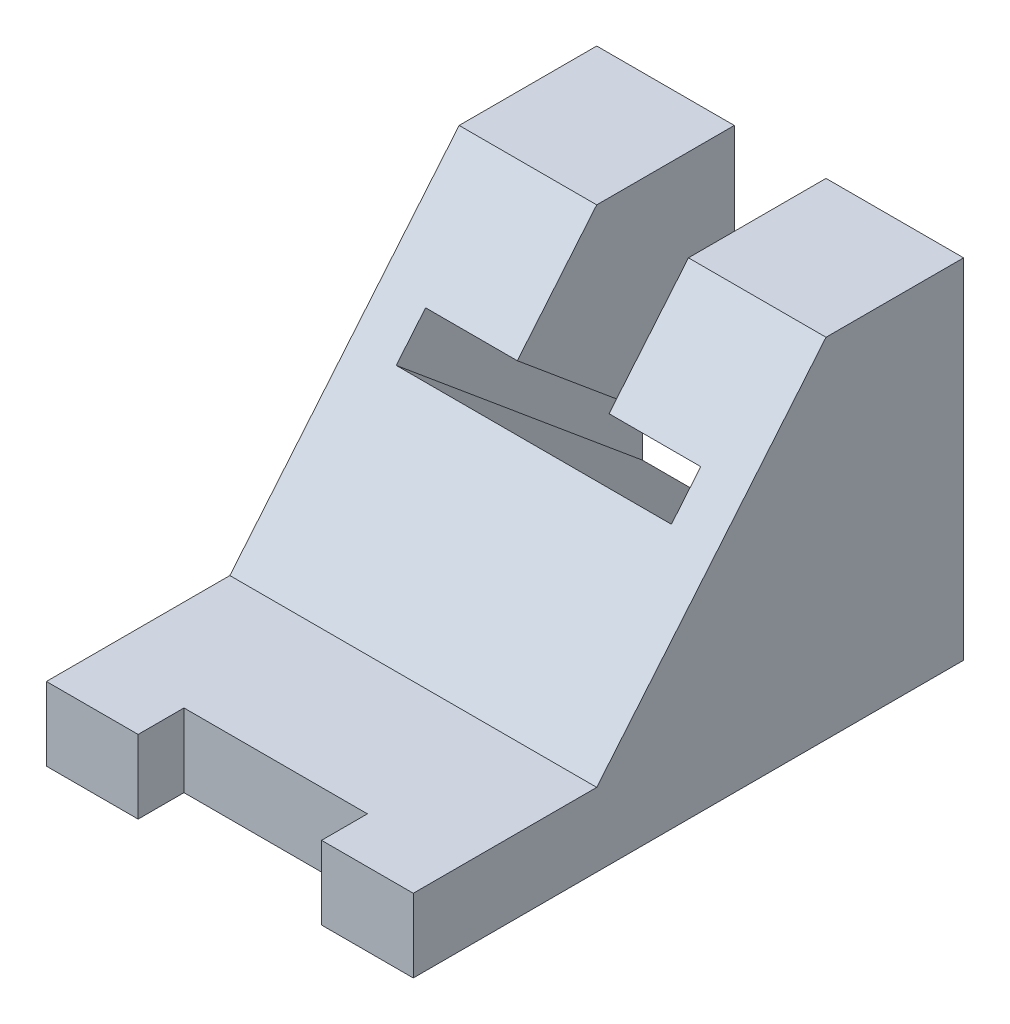
ISO-10303-21;
HEADER;
FILE_DESCRIPTION(('STEP AP214'),'2;1');
FILE_NAME('part.step','',(''),(''),'','','');
FILE_SCHEMA(('AUTOMOTIVE_DESIGN { 1 0 10303 214 1 1 1 1 }'));
ENDSEC;
DATA;
#1=APPLICATION_CONTEXT('core data for automotive mechanical design processes');
#2=APPLICATION_PROTOCOL_DEFINITION('international standard','automotive_design',2000,#1);
#3=PRODUCT_CONTEXT('',#1,'mechanical');
#4=PRODUCT('Part','Part','',(#3));
#5=PRODUCT_RELATED_PRODUCT_CATEGORY('part','',(#4));
#6=PRODUCT_DEFINITION_FORMATION('','',#4);
#7=PRODUCT_DEFINITION_CONTEXT('part definition',#1,'design');
#8=PRODUCT_DEFINITION('design','',#6,#7);
#9=PRODUCT_DEFINITION_SHAPE('','',#8);
#10=(LENGTH_UNIT() NAMED_UNIT(*) SI_UNIT(.MILLI.,.METRE.));
#11=(NAMED_UNIT(*) PLANE_ANGLE_UNIT() SI_UNIT($,.RADIAN.));
#12=(NAMED_UNIT(*) SI_UNIT($,.STERADIAN.) SOLID_ANGLE_UNIT());
#13=UNCERTAINTY_MEASURE_WITH_UNIT(LENGTH_MEASURE(1.E-05),#10,'distance_accuracy_value','');
#14=(GEOMETRIC_REPRESENTATION_CONTEXT(3) GLOBAL_UNCERTAINTY_ASSIGNED_CONTEXT((#13)) GLOBAL_UNIT_ASSIGNED_CONTEXT((#10,
#11,#12)) REPRESENTATION_CONTEXT('',''));
#15=CARTESIAN_POINT('',(0.,0.,0.));
#16=DIRECTION('',(0.,0.,1.));
#17=DIRECTION('',(1.,0.,0.));
#18=AXIS2_PLACEMENT_3D('',#15,#16,#17);
#19=CARTESIAN_POINT('',(-20.,38.,-30.));
#20=DIRECTION('',(0.,1.,0.));
#21=DIRECTION('',(0.,0.,1.));
#22=AXIS2_PLACEMENT_3D('',#19,#20,#21);
#23=PLANE('',#22);
#24=DIRECTION('',(0.,0.,-1.));
#25=VECTOR('',#24,1.);
#26=CARTESIAN_POINT('',(5.,38.,-15.));
#27=LINE('',#26,#25);
#28=CARTESIAN_POINT('',(5.,38.,-15.));
#29=VERTEX_POINT('',#28);
#30=CARTESIAN_POINT('',(5.,38.,-30.));
#31=VERTEX_POINT('',#30);
#32=EDGE_CURVE('E187',#29,#31,#27,.T.);
#33=ORIENTED_EDGE('',*,*,#32,.F.);
#34=DIRECTION('',(1.,0.,0.));
#35=VECTOR('',#34,1.);
#36=CARTESIAN_POINT('',(-20.,38.,-15.));
#37=LINE('',#36,#35);
#38=CARTESIAN_POINT('',(20.,38.,-15.));
#39=VERTEX_POINT('',#38);
#40=EDGE_CURVE('E275',#29,#39,#37,.T.);
#41=ORIENTED_EDGE('',*,*,#40,.T.);
#42=DIRECTION('',(0.,0.,1.));
#43=VECTOR('',#42,1.);
#44=CARTESIAN_POINT('',(20.,38.,-30.));
#45=LINE('',#44,#43);
#46=CARTESIAN_POINT('',(20.,38.,-30.));
#47=VERTEX_POINT('',#46);
#48=EDGE_CURVE('E269',#47,#39,#45,.T.);
#49=ORIENTED_EDGE('',*,*,#48,.F.);
#50=DIRECTION('',(1.,0.,0.));
#51=VECTOR('',#50,1.);
#52=CARTESIAN_POINT('',(-20.,38.,-30.));
#53=LINE('',#52,#51);
#54=EDGE_CURVE('E195',#31,#47,#53,.T.);
#55=ORIENTED_EDGE('',*,*,#54,.F.);
#56=EDGE_LOOP('',(#33,#41,#49,#55));
#57=FACE_BOUND('',#56,.T.);
#58=ADVANCED_FACE('F39',(#57),#23,.T.);
#59=CARTESIAN_POINT('',(20.,8.,30.));
#60=DIRECTION('',(0.,0.,-1.));
#61=DIRECTION('',(-1.,0.,0.));
#62=AXIS2_PLACEMENT_3D('',#59,#60,#61);
#63=PLANE('',#62);
#64=DIRECTION('',(1.,0.,0.));
#65=VECTOR('',#64,1.);
#66=CARTESIAN_POINT('',(20.,8.,30.));
#67=LINE('',#66,#65);
#68=CARTESIAN_POINT('',(10.,8.,30.));
#69=VERTEX_POINT('',#68);
#70=CARTESIAN_POINT('',(20.,8.,30.));
#71=VERTEX_POINT('',#70);
#72=EDGE_CURVE('E217',#69,#71,#67,.T.);
#73=ORIENTED_EDGE('',*,*,#72,.F.);
#74=DIRECTION('',(0.,1.,0.));
#75=VECTOR('',#74,1.);
#76=CARTESIAN_POINT('',(10.,-12.,30.));
#77=LINE('',#76,#75);
#78=CARTESIAN_POINT('',(10.,0.,30.));
#79=VERTEX_POINT('',#78);
#80=EDGE_CURVE('E210',#79,#69,#77,.T.);
#81=ORIENTED_EDGE('',*,*,#80,.F.);
#82=DIRECTION('',(1.,0.,0.));
#83=VECTOR('',#82,1.);
#84=CARTESIAN_POINT('',(20.,0.,30.));
#85=LINE('',#84,#83);
#86=CARTESIAN_POINT('',(20.,0.,30.));
#87=VERTEX_POINT('',#86);
#88=EDGE_CURVE('E226',#79,#87,#85,.T.);
#89=ORIENTED_EDGE('',*,*,#88,.T.);
#90=DIRECTION('',(0.,-1.,0.));
#91=VECTOR('',#90,1.);
#92=CARTESIAN_POINT('',(20.,8.,30.));
#93=LINE('',#92,#91);
#94=EDGE_CURVE('E237',#71,#87,#93,.T.);
#95=ORIENTED_EDGE('',*,*,#94,.F.);
#96=EDGE_LOOP('',(#73,#81,#89,#95));
#97=FACE_BOUND('',#96,.T.);
#98=ADVANCED_FACE('F342',(#97),#63,.F.);
#99=CARTESIAN_POINT('',(-20.,8.,30.));
#100=DIRECTION('',(1.,0.,0.));
#101=DIRECTION('',(0.,0.,-1.));
#102=AXIS2_PLACEMENT_3D('',#99,#100,#101);
#103=PLANE('',#102);
#104=DIRECTION('',(0.,0.,1.));
#105=VECTOR('',#104,1.);
#106=CARTESIAN_POINT('',(-20.,8.,30.));
#107=LINE('',#106,#105);
#108=CARTESIAN_POINT('',(-20.,8.,9.99999999999999));
#109=VERTEX_POINT('',#108);
#110=CARTESIAN_POINT('',(-20.,8.,30.));
#111=VERTEX_POINT('',#110);
#112=EDGE_CURVE('E216',#109,#111,#107,.T.);
#113=ORIENTED_EDGE('',*,*,#112,.F.);
#114=DIRECTION('',(0.,0.768221279597376,-0.64018439966448));
#115=VECTOR('',#114,1.);
#116=CARTESIAN_POINT('',(-20.,38.,-15.));
#117=LINE('',#116,#115);
#118=CARTESIAN_POINT('',(-20.,38.,-15.));
#119=VERTEX_POINT('',#118);
#120=EDGE_CURVE('E276',#109,#119,#117,.T.);
#121=ORIENTED_EDGE('',*,*,#120,.T.);
#122=DIRECTION('',(0.,0.,1.));
#123=VECTOR('',#122,1.);
#124=CARTESIAN_POINT('',(-20.,38.,-30.));
#125=LINE('',#124,#123);
#126=CARTESIAN_POINT('',(-20.,38.,-30.));
#127=VERTEX_POINT('',#126);
#128=EDGE_CURVE('E196',#127,#119,#125,.T.);
#129=ORIENTED_EDGE('',*,*,#128,.F.);
#130=DIRECTION('',(0.,-1.,0.));
#131=VECTOR('',#130,1.);
#132=CARTESIAN_POINT('',(-20.,8.,-30.));
#133=LINE('',#132,#131);
#134=CARTESIAN_POINT('',(-20.,0.,-30.));
#135=VERTEX_POINT('',#134);
#136=EDGE_CURVE('E188',#127,#135,#133,.T.);
#137=ORIENTED_EDGE('',*,*,#136,.T.);
#138=DIRECTION('',(0.,0.,1.));
#139=VECTOR('',#138,1.);
#140=CARTESIAN_POINT('',(-20.,0.,30.));
#141=LINE('',#140,#139);
#142=CARTESIAN_POINT('',(-20.,0.,30.));
#143=VERTEX_POINT('',#142);
#144=EDGE_CURVE('E209',#135,#143,#141,.T.);
#145=ORIENTED_EDGE('',*,*,#144,.T.);
#146=DIRECTION('',(0.,-1.,0.));
#147=VECTOR('',#146,1.);
#148=CARTESIAN_POINT('',(-20.,8.,30.));
#149=LINE('',#148,#147);
#150=EDGE_CURVE('E245',#111,#143,#149,.T.);
#151=ORIENTED_EDGE('',*,*,#150,.F.);
#152=EDGE_LOOP('',(#113,#121,#129,#137,#145,#151));
#153=FACE_BOUND('',#152,.T.);
#154=ADVANCED_FACE('F41',(#153),#103,.F.);
#155=CARTESIAN_POINT('',(-10.,0.,30.));
#156=VERTEX_POINT('',#155);
#157=EDGE_CURVE('E230',#143,#156,#85,.T.);
#158=ORIENTED_EDGE('',*,*,#157,.T.);
#159=DIRECTION('',(0.,1.,0.));
#160=VECTOR('',#159,1.);
#161=CARTESIAN_POINT('',(-10.,-12.,30.));
#162=LINE('',#161,#160);
#163=CARTESIAN_POINT('',(-10.,8.,30.));
#164=VERTEX_POINT('',#163);
#165=EDGE_CURVE('E208',#156,#164,#162,.T.);
#166=ORIENTED_EDGE('',*,*,#165,.T.);
#167=EDGE_CURVE('E219',#111,#164,#67,.T.);
#168=ORIENTED_EDGE('',*,*,#167,.F.);
#169=ORIENTED_EDGE('',*,*,#150,.T.);
#170=EDGE_LOOP('',(#158,#166,#168,#169));
#171=FACE_BOUND('',#170,.T.);
#172=ADVANCED_FACE('F253',(#171),#63,.F.);
#173=CARTESIAN_POINT('',(20.,8.,30.));
#174=DIRECTION('',(-1.,0.,0.));
#175=DIRECTION('',(0.,0.,1.));
#176=AXIS2_PLACEMENT_3D('',#173,#174,#175);
#177=PLANE('',#176);
#178=ORIENTED_EDGE('',*,*,#48,.T.);
#179=DIRECTION('',(0.,0.768221279597376,-0.64018439966448));
#180=VECTOR('',#179,1.);
#181=CARTESIAN_POINT('',(20.,38.,-15.));
#182=LINE('',#181,#180);
#183=CARTESIAN_POINT('',(20.,8.,9.99999999999999));
#184=VERTEX_POINT('',#183);
#185=EDGE_CURVE('E280',#184,#39,#182,.T.);
#186=ORIENTED_EDGE('',*,*,#185,.F.);
#187=DIRECTION('',(0.,0.,-1.));
#188=VECTOR('',#187,1.);
#189=CARTESIAN_POINT('',(20.,8.,30.));
#190=LINE('',#189,#188);
#191=EDGE_CURVE('E221',#71,#184,#190,.T.);
#192=ORIENTED_EDGE('',*,*,#191,.F.);
#193=ORIENTED_EDGE('',*,*,#94,.T.);
#194=DIRECTION('',(0.,0.,-1.));
#195=VECTOR('',#194,1.);
#196=CARTESIAN_POINT('',(20.,0.,30.));
#197=LINE('',#196,#195);
#198=CARTESIAN_POINT('',(20.,0.,-30.));
#199=VERTEX_POINT('',#198);
#200=EDGE_CURVE('E235',#87,#199,#197,.T.);
#201=ORIENTED_EDGE('',*,*,#200,.T.);
#202=DIRECTION('',(0.,-1.,0.));
#203=VECTOR('',#202,1.);
#204=CARTESIAN_POINT('',(20.,8.,-30.));
#205=LINE('',#204,#203);
#206=EDGE_CURVE('E236',#47,#199,#205,.T.);
#207=ORIENTED_EDGE('',*,*,#206,.F.);
#208=EDGE_LOOP('',(#178,#186,#192,#193,#201,#207));
#209=FACE_BOUND('',#208,.T.);
#210=ADVANCED_FACE('F270',(#209),#177,.F.);
#211=CARTESIAN_POINT('',(20.,8.,-30.));
#212=DIRECTION('',(0.,0.,1.));
#213=DIRECTION('',(1.,0.,0.));
#214=AXIS2_PLACEMENT_3D('',#211,#212,#213);
#215=PLANE('',#214);
#216=DIRECTION('',(0.,1.,0.));
#217=VECTOR('',#216,1.);
#218=CARTESIAN_POINT('',(5.,8.,-30.));
#219=LINE('',#218,#217);
#220=CARTESIAN_POINT('',(5.,7.8976526277451,-30.));
#221=VERTEX_POINT('',#220);
#222=EDGE_CURVE('E176',#221,#31,#219,.T.);
#223=ORIENTED_EDGE('',*,*,#222,.T.);
#224=ORIENTED_EDGE('',*,*,#54,.T.);
#225=ORIENTED_EDGE('',*,*,#206,.T.);
#226=DIRECTION('',(-1.,0.,0.));
#227=VECTOR('',#226,1.);
#228=CARTESIAN_POINT('',(20.,0.,-30.));
#229=LINE('',#228,#227);
#230=EDGE_CURVE('E218',#199,#135,#229,.T.);
#231=ORIENTED_EDGE('',*,*,#230,.T.);
#232=ORIENTED_EDGE('',*,*,#136,.F.);
#233=CARTESIAN_POINT('',(-5.,38.,-30.));
#234=VERTEX_POINT('',#233);
#235=EDGE_CURVE('E182',#127,#234,#53,.T.);
#236=ORIENTED_EDGE('',*,*,#235,.T.);
#237=DIRECTION('',(0.,-1.,0.));
#238=VECTOR('',#237,1.);
#239=CARTESIAN_POINT('',(-5.,8.,-30.));
#240=LINE('',#239,#238);
#241=CARTESIAN_POINT('',(-5.,7.8976526277451,-30.));
#242=VERTEX_POINT('',#241);
#243=EDGE_CURVE('E164',#234,#242,#240,.T.);
#244=ORIENTED_EDGE('',*,*,#243,.T.);
#245=DIRECTION('',(-1.,0.,0.));
#246=VECTOR('',#245,1.);
#247=CARTESIAN_POINT('',(20.,7.89765262774512,-30.));
#248=LINE('',#247,#246);
#249=CARTESIAN_POINT('',(-15.,7.89765262774509,-30.));
#250=VERTEX_POINT('',#249);
#251=EDGE_CURVE('E174',#242,#250,#248,.T.);
#252=ORIENTED_EDGE('',*,*,#251,.T.);
#253=DIRECTION('',(0.,-1.,0.));
#254=VECTOR('',#253,1.);
#255=CARTESIAN_POINT('',(-15.,7.99999999999999,-30.));
#256=LINE('',#255,#254);
#257=CARTESIAN_POINT('',(-15.,1.38911123115622,-30.));
#258=VERTEX_POINT('',#257);
#259=EDGE_CURVE('E286',#250,#258,#256,.T.);
#260=ORIENTED_EDGE('',*,*,#259,.T.);
#261=DIRECTION('',(1.,0.,0.));
#262=VECTOR('',#261,1.);
#263=CARTESIAN_POINT('',(20.,1.38911123115622,-30.));
#264=LINE('',#263,#262);
#265=CARTESIAN_POINT('',(15.,1.38911123115622,-30.));
#266=VERTEX_POINT('',#265);
#267=EDGE_CURVE('E284',#258,#266,#264,.T.);
#268=ORIENTED_EDGE('',*,*,#267,.T.);
#269=DIRECTION('',(0.,1.,0.));
#270=VECTOR('',#269,1.);
#271=CARTESIAN_POINT('',(15.,8.,-30.));
#272=LINE('',#271,#270);
#273=CARTESIAN_POINT('',(15.,7.8976526277451,-30.));
#274=VERTEX_POINT('',#273);
#275=EDGE_CURVE('E278',#266,#274,#272,.T.);
#276=ORIENTED_EDGE('',*,*,#275,.T.);
#277=DIRECTION('',(-1.,0.,0.));
#278=VECTOR('',#277,1.);
#279=CARTESIAN_POINT('',(20.,7.8976526277451,-30.));
#280=LINE('',#279,#278);
#281=EDGE_CURVE('E291',#274,#221,#280,.T.);
#282=ORIENTED_EDGE('',*,*,#281,.T.);
#283=EDGE_LOOP('',(#223,#224,#225,#231,#232,#236,#244,#252,#260,#268,#276,#282));
#284=FACE_BOUND('',#283,.T.);
#285=ADVANCED_FACE('F189',(#284),#215,.F.);
#286=CARTESIAN_POINT('',(0.,8.,0.));
#287=DIRECTION('',(0.,1.,0.));
#288=DIRECTION('',(0.,0.,1.));
#289=AXIS2_PLACEMENT_3D('',#286,#287,#288);
#290=PLANE('',#289);
#291=DIRECTION('',(1.,0.,0.));
#292=VECTOR('',#291,1.);
#293=CARTESIAN_POINT('',(-20.,8.,9.99999999999999));
#294=LINE('',#293,#292);
#295=EDGE_CURVE('E192',#109,#184,#294,.T.);
#296=ORIENTED_EDGE('',*,*,#295,.F.);
#297=ORIENTED_EDGE('',*,*,#112,.T.);
#298=ORIENTED_EDGE('',*,*,#167,.T.);
#299=DIRECTION('',(0.,0.,1.));
#300=VECTOR('',#299,1.);
#301=CARTESIAN_POINT('',(-10.,8.,30.));
#302=LINE('',#301,#300);
#303=CARTESIAN_POINT('',(-10.,8.,25.));
#304=VERTEX_POINT('',#303);
#305=EDGE_CURVE('E204',#304,#164,#302,.T.);
#306=ORIENTED_EDGE('',*,*,#305,.F.);
#307=DIRECTION('',(-1.,0.,0.));
#308=VECTOR('',#307,1.);
#309=CARTESIAN_POINT('',(-10.,8.,25.));
#310=LINE('',#309,#308);
#311=CARTESIAN_POINT('',(10.,8.,25.));
#312=VERTEX_POINT('',#311);
#313=EDGE_CURVE('E203',#312,#304,#310,.T.);
#314=ORIENTED_EDGE('',*,*,#313,.F.);
#315=DIRECTION('',(0.,0.,-1.));
#316=VECTOR('',#315,1.);
#317=CARTESIAN_POINT('',(10.,8.,30.));
#318=LINE('',#317,#316);
#319=EDGE_CURVE('E191',#69,#312,#318,.T.);
#320=ORIENTED_EDGE('',*,*,#319,.F.);
#321=ORIENTED_EDGE('',*,*,#72,.T.);
#322=ORIENTED_EDGE('',*,*,#191,.T.);
#323=EDGE_LOOP('',(#296,#297,#298,#306,#314,#320,#321,#322));
#324=FACE_BOUND('',#323,.T.);
#325=ADVANCED_FACE('F334',(#324),#290,.T.);
#326=CARTESIAN_POINT('',(0.,0.,0.));
#327=DIRECTION('',(0.,1.,0.));
#328=DIRECTION('',(0.,0.,1.));
#329=AXIS2_PLACEMENT_3D('',#326,#327,#328);
#330=PLANE('',#329);
#331=ORIENTED_EDGE('',*,*,#88,.F.);
#332=DIRECTION('',(0.,0.,-1.));
#333=VECTOR('',#332,1.);
#334=CARTESIAN_POINT('',(10.,0.,0.));
#335=LINE('',#334,#333);
#336=CARTESIAN_POINT('',(10.,0.,25.));
#337=VERTEX_POINT('',#336);
#338=EDGE_CURVE('E11',#79,#337,#335,.T.);
#339=ORIENTED_EDGE('',*,*,#338,.T.);
#340=DIRECTION('',(-1.,0.,0.));
#341=VECTOR('',#340,1.);
#342=CARTESIAN_POINT('',(0.,0.,25.));
#343=LINE('',#342,#341);
#344=CARTESIAN_POINT('',(-10.,0.,25.));
#345=VERTEX_POINT('',#344);
#346=EDGE_CURVE('E244',#337,#345,#343,.T.);
#347=ORIENTED_EDGE('',*,*,#346,.T.);
#348=DIRECTION('',(0.,0.,1.));
#349=VECTOR('',#348,1.);
#350=CARTESIAN_POINT('',(-10.,0.,0.));
#351=LINE('',#350,#349);
#352=EDGE_CURVE('E50',#345,#156,#351,.T.);
#353=ORIENTED_EDGE('',*,*,#352,.T.);
#354=ORIENTED_EDGE('',*,*,#157,.F.);
#355=ORIENTED_EDGE('',*,*,#144,.F.);
#356=ORIENTED_EDGE('',*,*,#230,.F.);
#357=ORIENTED_EDGE('',*,*,#200,.F.);
#358=EDGE_LOOP('',(#331,#339,#347,#353,#354,#355,#356,#357));
#359=FACE_BOUND('',#358,.T.);
#360=ADVANCED_FACE('F252',(#359),#330,.F.);
#361=CARTESIAN_POINT('',(10.,-12.,30.));
#362=DIRECTION('',(1.,0.,0.));
#363=DIRECTION('',(0.,0.,-1.));
#364=AXIS2_PLACEMENT_3D('',#361,#362,#363);
#365=PLANE('',#364);
#366=ORIENTED_EDGE('',*,*,#80,.T.);
#367=ORIENTED_EDGE('',*,*,#319,.T.);
#368=DIRECTION('',(0.,1.,0.));
#369=VECTOR('',#368,1.);
#370=CARTESIAN_POINT('',(10.,-12.,25.));
#371=LINE('',#370,#369);
#372=EDGE_CURVE('E207',#337,#312,#371,.T.);
#373=ORIENTED_EDGE('',*,*,#372,.F.);
#374=ORIENTED_EDGE('',*,*,#338,.F.);
#375=EDGE_LOOP('',(#366,#367,#373,#374));
#376=FACE_BOUND('',#375,.T.);
#377=ADVANCED_FACE('F341',(#376),#365,.F.);
#378=CARTESIAN_POINT('',(-10.,-12.,30.));
#379=DIRECTION('',(-1.,0.,0.));
#380=DIRECTION('',(0.,0.,1.));
#381=AXIS2_PLACEMENT_3D('',#378,#379,#380);
#382=PLANE('',#381);
#383=DIRECTION('',(0.,1.,0.));
#384=VECTOR('',#383,1.);
#385=CARTESIAN_POINT('',(-10.,-12.,25.));
#386=LINE('',#385,#384);
#387=EDGE_CURVE('E214',#345,#304,#386,.T.);
#388=ORIENTED_EDGE('',*,*,#387,.T.);
#389=ORIENTED_EDGE('',*,*,#305,.T.);
#390=ORIENTED_EDGE('',*,*,#165,.F.);
#391=ORIENTED_EDGE('',*,*,#352,.F.);
#392=EDGE_LOOP('',(#388,#389,#390,#391));
#393=FACE_BOUND('',#392,.T.);
#394=ADVANCED_FACE('F347',(#393),#382,.F.);
#395=CARTESIAN_POINT('',(-10.,-12.,25.));
#396=DIRECTION('',(0.,0.,-1.));
#397=DIRECTION('',(-1.,0.,0.));
#398=AXIS2_PLACEMENT_3D('',#395,#396,#397);
#399=PLANE('',#398);
#400=ORIENTED_EDGE('',*,*,#372,.T.);
#401=ORIENTED_EDGE('',*,*,#313,.T.);
#402=ORIENTED_EDGE('',*,*,#387,.F.);
#403=ORIENTED_EDGE('',*,*,#346,.F.);
#404=EDGE_LOOP('',(#400,#401,#402,#403));
#405=FACE_BOUND('',#404,.T.);
#406=ADVANCED_FACE('F346',(#405),#399,.F.);
#407=DIRECTION('',(0.,0.,1.));
#408=VECTOR('',#407,1.);
#409=CARTESIAN_POINT('',(-5.,38.,-15.));
#410=LINE('',#409,#408);
#411=CARTESIAN_POINT('',(-5.,38.,-15.));
#412=VERTEX_POINT('',#411);
#413=EDGE_CURVE('E169',#234,#412,#410,.T.);
#414=ORIENTED_EDGE('',*,*,#413,.F.);
#415=ORIENTED_EDGE('',*,*,#235,.F.);
#416=ORIENTED_EDGE('',*,*,#128,.T.);
#417=EDGE_CURVE('E184',#119,#412,#37,.T.);
#418=ORIENTED_EDGE('',*,*,#417,.T.);
#419=EDGE_LOOP('',(#414,#415,#416,#418));
#420=FACE_BOUND('',#419,.T.);
#421=ADVANCED_FACE('F181',(#420),#23,.T.);
#422=CARTESIAN_POINT('',(-20.,38.,-15.));
#423=DIRECTION('',(0.,-0.64018439966448,-0.768221279597376));
#424=DIRECTION('',(0.,0.768221279597376,-0.64018439966448));
#425=AXIS2_PLACEMENT_3D('',#422,#423,#424);
#426=PLANE('',#425);
#427=DIRECTION('',(-1.,0.,0.));
#428=VECTOR('',#427,1.);
#429=CARTESIAN_POINT('',(-5.,27.6117294196528,-6.34310784971071));
#430=LINE('',#429,#428);
#431=CARTESIAN_POINT('',(-5.,27.6117294196528,-6.34310784971071));
#432=VERTEX_POINT('',#431);
#433=CARTESIAN_POINT('',(-15.,27.6117294196528,-6.34310784971071));
#434=VERTEX_POINT('',#433);
#435=EDGE_CURVE('E315',#432,#434,#430,.T.);
#436=ORIENTED_EDGE('',*,*,#435,.F.);
#437=DIRECTION('',(0.,-0.768221279597376,0.64018439966448));
#438=VECTOR('',#437,1.);
#439=CARTESIAN_POINT('',(-5.,38.,-15.));
#440=LINE('',#439,#438);
#441=EDGE_CURVE('E314',#412,#432,#440,.T.);
#442=ORIENTED_EDGE('',*,*,#441,.F.);
#443=ORIENTED_EDGE('',*,*,#417,.F.);
#444=ORIENTED_EDGE('',*,*,#120,.F.);
#445=ORIENTED_EDGE('',*,*,#295,.T.);
#446=ORIENTED_EDGE('',*,*,#185,.T.);
#447=ORIENTED_EDGE('',*,*,#40,.F.);
#448=DIRECTION('',(0.,0.768221279597376,-0.64018439966448));
#449=VECTOR('',#448,1.);
#450=CARTESIAN_POINT('',(5.,38.,-15.));
#451=LINE('',#450,#449);
#452=CARTESIAN_POINT('',(5.,27.6117294196528,-6.34310784971071));
#453=VERTEX_POINT('',#452);
#454=EDGE_CURVE('E320',#453,#29,#451,.T.);
#455=ORIENTED_EDGE('',*,*,#454,.F.);
#456=DIRECTION('',(-1.,0.,0.));
#457=VECTOR('',#456,1.);
#458=CARTESIAN_POINT('',(15.,27.6117294196528,-6.34310784971071));
#459=LINE('',#458,#457);
#460=CARTESIAN_POINT('',(15.,27.6117294196528,-6.34310784971072));
#461=VERTEX_POINT('',#460);
#462=EDGE_CURVE('E318',#461,#453,#459,.T.);
#463=ORIENTED_EDGE('',*,*,#462,.F.);
#464=DIRECTION('',(0.,0.768221279597376,-0.640184399664479));
#465=VECTOR('',#464,1.);
#466=CARTESIAN_POINT('',(15.,23.770623021666,-3.14218585138831));
#467=LINE('',#466,#465);
#468=CARTESIAN_POINT('',(15.,23.770623021666,-3.14218585138831));
#469=VERTEX_POINT('',#468);
#470=EDGE_CURVE('E65',#469,#461,#467,.T.);
#471=ORIENTED_EDGE('',*,*,#470,.F.);
#472=DIRECTION('',(1.,0.,0.));
#473=VECTOR('',#472,1.);
#474=CARTESIAN_POINT('',(-15.,23.770623021666,-3.14218585138831));
#475=LINE('',#474,#473);
#476=CARTESIAN_POINT('',(-15.,23.770623021666,-3.14218585138831));
#477=VERTEX_POINT('',#476);
#478=EDGE_CURVE('E299',#477,#469,#475,.T.);
#479=ORIENTED_EDGE('',*,*,#478,.F.);
#480=DIRECTION('',(0.,-0.768221279597375,0.64018439966448));
#481=VECTOR('',#480,1.);
#482=CARTESIAN_POINT('',(-15.,27.6117294196528,-6.34310784971071));
#483=LINE('',#482,#481);
#484=EDGE_CURVE('E307',#434,#477,#483,.T.);
#485=ORIENTED_EDGE('',*,*,#484,.F.);
#486=EDGE_LOOP('',(#436,#442,#443,#444,#445,#446,#447,#455,#463,#471,#479,#485));
#487=FACE_BOUND('',#486,.T.);
#488=ADVANCED_FACE('F329',(#487),#426,.F.);
#489=CARTESIAN_POINT('',(15.,-1.19656856524876,-33.102815755686));
#490=DIRECTION('',(1.,0.,0.));
#491=DIRECTION('',(0.,1.,0.));
#492=AXIS2_PLACEMENT_3D('',#489,#490,#491);
#493=PLANE('',#492);
#494=DIRECTION('',(0.,0.64018439966448,0.768221279597376));
#495=VECTOR('',#494,1.);
#496=CARTESIAN_POINT('',(15.,-1.19656856524876,-33.102815755686));
#497=LINE('',#496,#495);
#498=EDGE_CURVE('E298',#266,#469,#497,.T.);
#499=ORIENTED_EDGE('',*,*,#498,.T.);
#500=ORIENTED_EDGE('',*,*,#470,.T.);
#501=DIRECTION('',(0.,0.64018439966448,0.768221279597376));
#502=VECTOR('',#501,1.);
#503=CARTESIAN_POINT('',(15.,2.64453783273812,-36.3037377540084));
#504=LINE('',#503,#502);
#505=EDGE_CURVE('E300',#274,#461,#504,.T.);
#506=ORIENTED_EDGE('',*,*,#505,.F.);
#507=ORIENTED_EDGE('',*,*,#275,.F.);
#508=EDGE_LOOP('',(#499,#500,#506,#507));
#509=FACE_BOUND('',#508,.T.);
#510=ADVANCED_FACE('F359',(#509),#493,.F.);
#511=CARTESIAN_POINT('',(-15.,-1.19656856524876,-33.102815755686));
#512=DIRECTION('',(0.,-0.768221279597376,0.64018439966448));
#513=DIRECTION('',(0.,-0.64018439966448,-0.768221279597376));
#514=AXIS2_PLACEMENT_3D('',#511,#512,#513);
#515=PLANE('',#514);
#516=DIRECTION('',(0.,0.64018439966448,0.768221279597376));
#517=VECTOR('',#516,1.);
#518=CARTESIAN_POINT('',(-15.,-1.19656856524876,-33.102815755686));
#519=LINE('',#518,#517);
#520=EDGE_CURVE('E302',#258,#477,#519,.T.);
#521=ORIENTED_EDGE('',*,*,#520,.T.);
#522=ORIENTED_EDGE('',*,*,#478,.T.);
#523=ORIENTED_EDGE('',*,*,#498,.F.);
#524=ORIENTED_EDGE('',*,*,#267,.F.);
#525=EDGE_LOOP('',(#521,#522,#523,#524));
#526=FACE_BOUND('',#525,.T.);
#527=ADVANCED_FACE('F356',(#526),#515,.F.);
#528=CARTESIAN_POINT('',(-15.,2.64453783273812,-36.3037377540084));
#529=DIRECTION('',(-1.,0.,0.));
#530=DIRECTION('',(0.,-1.,0.));
#531=AXIS2_PLACEMENT_3D('',#528,#529,#530);
#532=PLANE('',#531);
#533=DIRECTION('',(0.,0.64018439966448,0.768221279597376));
#534=VECTOR('',#533,1.);
#535=CARTESIAN_POINT('',(-15.,2.64453783273812,-36.3037377540084));
#536=LINE('',#535,#534);
#537=EDGE_CURVE('E305',#250,#434,#536,.T.);
#538=ORIENTED_EDGE('',*,*,#537,.T.);
#539=ORIENTED_EDGE('',*,*,#484,.T.);
#540=ORIENTED_EDGE('',*,*,#520,.F.);
#541=ORIENTED_EDGE('',*,*,#259,.F.);
#542=EDGE_LOOP('',(#538,#539,#540,#541));
#543=FACE_BOUND('',#542,.T.);
#544=ADVANCED_FACE('F358',(#543),#532,.F.);
#545=CARTESIAN_POINT('',(-5.,2.64453783273812,-36.3037377540084));
#546=DIRECTION('',(0.,0.768221279597376,-0.64018439966448));
#547=DIRECTION('',(0.,0.64018439966448,0.768221279597376));
#548=AXIS2_PLACEMENT_3D('',#545,#546,#547);
#549=PLANE('',#548);
#550=DIRECTION('',(0.,0.64018439966448,0.768221279597376));
#551=VECTOR('',#550,1.);
#552=CARTESIAN_POINT('',(-5.,2.64453783273812,-36.3037377540084));
#553=LINE('',#552,#551);
#554=EDGE_CURVE('E171',#242,#432,#553,.T.);
#555=ORIENTED_EDGE('',*,*,#554,.T.);
#556=ORIENTED_EDGE('',*,*,#435,.T.);
#557=ORIENTED_EDGE('',*,*,#537,.F.);
#558=ORIENTED_EDGE('',*,*,#251,.F.);
#559=EDGE_LOOP('',(#555,#556,#557,#558));
#560=FACE_BOUND('',#559,.T.);
#561=ADVANCED_FACE('F351',(#560),#549,.F.);
#562=CARTESIAN_POINT('',(-5.,13.0328084130853,-44.9606299042977));
#563=DIRECTION('',(-1.,0.,0.));
#564=DIRECTION('',(0.,-1.,0.));
#565=AXIS2_PLACEMENT_3D('',#562,#563,#564);
#566=PLANE('',#565);
#567=ORIENTED_EDGE('',*,*,#243,.F.);
#568=ORIENTED_EDGE('',*,*,#413,.T.);
#569=ORIENTED_EDGE('',*,*,#441,.T.);
#570=ORIENTED_EDGE('',*,*,#554,.F.);
#571=EDGE_LOOP('',(#567,#568,#569,#570));
#572=FACE_BOUND('',#571,.T.);
#573=ADVANCED_FACE('F170',(#572),#566,.F.);
#574=CARTESIAN_POINT('',(5.,13.0328084130853,-44.9606299042977));
#575=DIRECTION('',(1.,0.,0.));
#576=DIRECTION('',(0.,1.,0.));
#577=AXIS2_PLACEMENT_3D('',#574,#575,#576);
#578=PLANE('',#577);
#579=DIRECTION('',(0.,0.64018439966448,0.768221279597376));
#580=VECTOR('',#579,1.);
#581=CARTESIAN_POINT('',(5.,2.64453783273812,-36.3037377540084));
#582=LINE('',#581,#580);
#583=EDGE_CURVE('E53',#221,#453,#582,.T.);
#584=ORIENTED_EDGE('',*,*,#583,.T.);
#585=ORIENTED_EDGE('',*,*,#454,.T.);
#586=ORIENTED_EDGE('',*,*,#32,.T.);
#587=ORIENTED_EDGE('',*,*,#222,.F.);
#588=EDGE_LOOP('',(#584,#585,#586,#587));
#589=FACE_BOUND('',#588,.T.);
#590=ADVANCED_FACE('F323',(#589),#578,.F.);
#591=CARTESIAN_POINT('',(15.,2.64453783273812,-36.3037377540084));
#592=DIRECTION('',(0.,0.768221279597376,-0.64018439966448));
#593=DIRECTION('',(0.,0.64018439966448,0.768221279597376));
#594=AXIS2_PLACEMENT_3D('',#591,#592,#593);
#595=PLANE('',#594);
#596=ORIENTED_EDGE('',*,*,#505,.T.);
#597=ORIENTED_EDGE('',*,*,#462,.T.);
#598=ORIENTED_EDGE('',*,*,#583,.F.);
#599=ORIENTED_EDGE('',*,*,#281,.F.);
#600=EDGE_LOOP('',(#596,#597,#598,#599));
#601=FACE_BOUND('',#600,.T.);
#602=ADVANCED_FACE('F363',(#601),#595,.F.);
#603=CLOSED_SHELL('',(#58,#98,#154,#172,#210,#285,#325,#360,#377,#394,#406,#421,#488,#510,#527,
#544,#561,#573,#590,#602));
#604=MANIFOLD_SOLID_BREP('B2',#603);
#605=ADVANCED_BREP_SHAPE_REPRESENTATION('',(#18,#604),#14);
#606=SHAPE_DEFINITION_REPRESENTATION(#9,#605);
ENDSEC;
END-ISO-10303-21;
